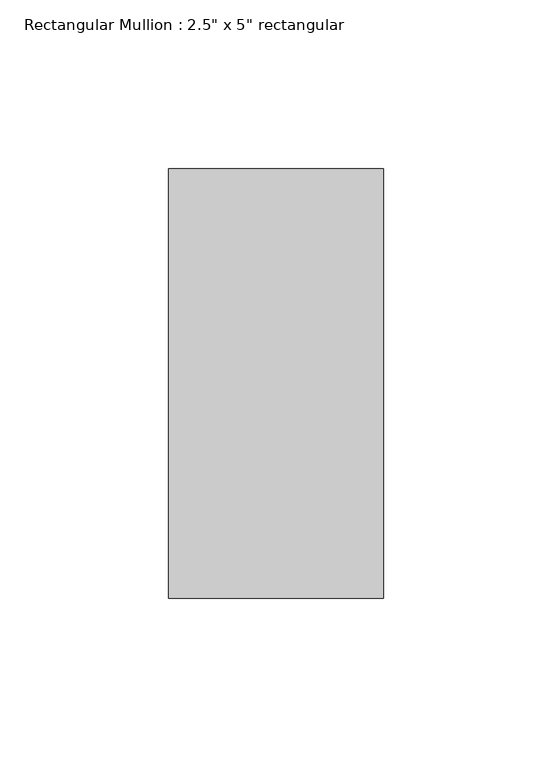
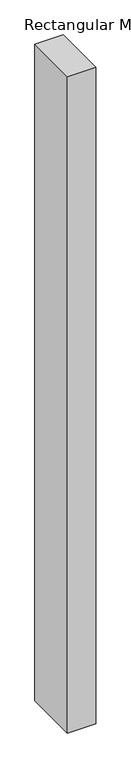
"""IFC4 building model written with IfcOpenShell, lengths in millimetres: member geometry."""

from ifc_helpers import new_model, si_unit, frame, origin, place, context, project, spatial, polyline, outline, extrude, source, transform, mapped, element, save


def member_fb9f8cdf(model_context):
    return source(origin(), model_context, "Body", "SweptSolid", [
        extrude(outline(polyline([(0.0, 63.5), (0.0, -63.5), (-63.5, -63.5), (-63.5, 63.5), (0.0, 63.5)])), frame((0.0, 0.0, -1562.1313909), z_axis=(0.0, 0.0, 1.0), x_axis=(1.0, 0.0, 0.0)), (0.0, 0.0, 1.0), 1562.1313909),
    ])


if __name__ == "__main__":
    model = new_model("IFC4")
    model_context = context("Model", 3, world=origin())
    ifc_project = project(units=[si_unit("LENGTHUNIT", "METRE", prefix="MILLI")], contexts=[model_context])
    site = spatial("IfcSite", under=ifc_project)
    building = spatial("IfcBuilding", under=site)
    placement = place(None, origin())
    member_shape = member_fb9f8cdf(model_context)
    element("IfcMember", 1, ObjectType="Rectangular Mullion : 2.5\" x 5\" rectangular", at=placement, inside=building, context=model_context, shape_type="MappedRepresentation", body=[
        mapped(member_shape, transform((0.0, 0.0, 0.0), x_axis=(1.0, 0.0, 0.0), y_axis=(0.0, 1.0, 0.0), z_axis=(0.0, 0.0, 1.0))),
    ])
    save(model, "model.ifc")

# Revit data of these elements
# Type "Rectangular Mullion : 2.5\" x 5\" rectangular"
#   built-in parameter 1007304 = 0.416667 (stored number, unit not read)
#   built-in parameter 1007301 = 0.104167 (stored number, unit not read)
#   built-in parameter 1007300 = 0.104167 (stored number, unit not read)
# Element 1 (IfcMember, "Rectangular Mullion : 2.5\" x 5\" rectangular")
#   Materials on its faces: "Aluminum"
# Materials
#   "Aluminum": class "Metal", colour RGB 247 247 247, transparency 0, Description = "Aluminum 6061", Cost = 0
